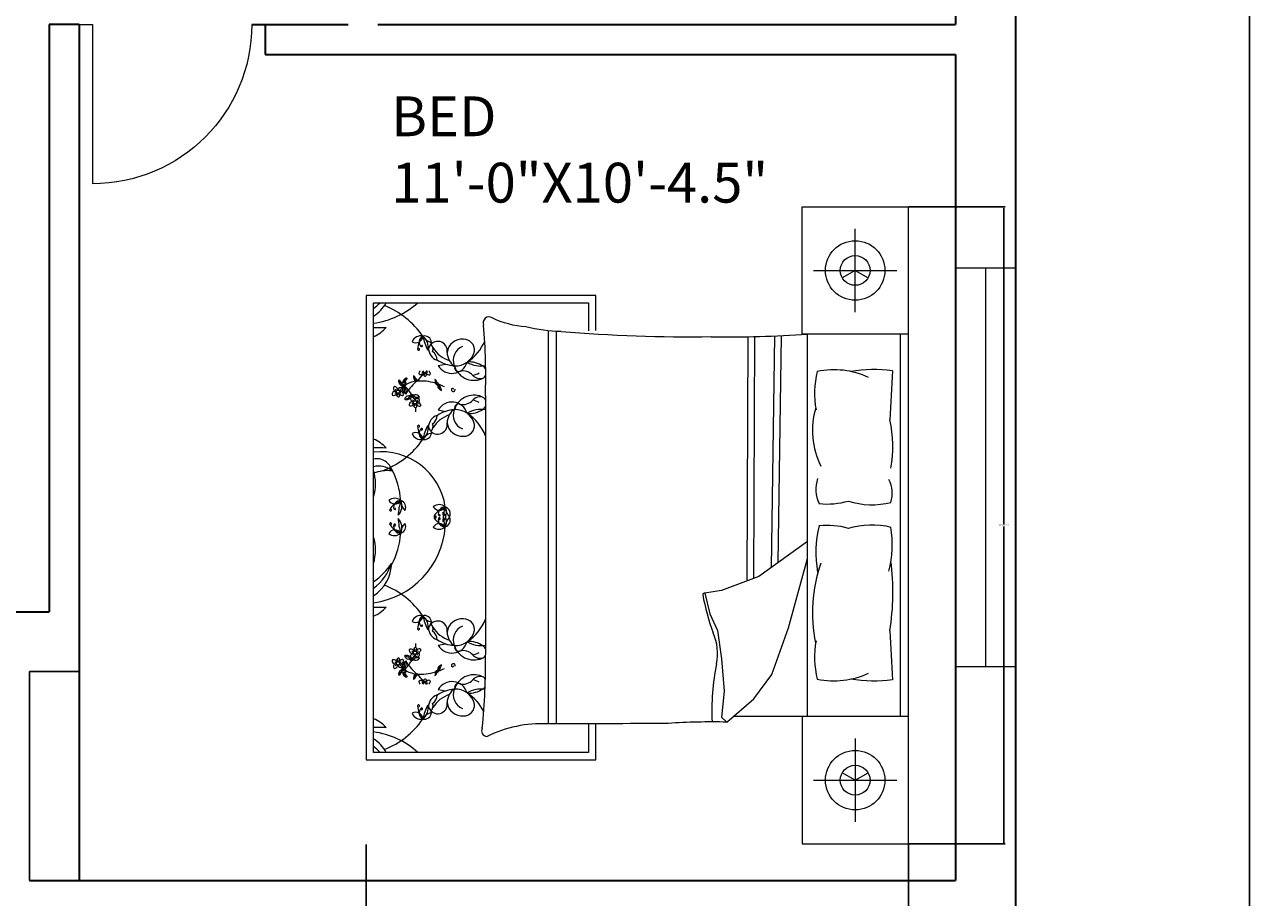
# Model space of a CAD drawing. Units: inches. Extents: x -59 to 444, y -680 to 63.
# Tile 8 of 9: x 260 to 444, y -306 to -175. Entities that reach past the tile are written whole.
import ezdxf

# ---------------------------------------------------------------- set-up
doc = ezdxf.new("R2010")
doc.units = ezdxf.units.IN
doc.header["$MEASUREMENT"] = 0
for name, color, linetype, lineweight in [('A-ANNO-DIMS', 2, 'Continuous', 18), ('A-AREA-IDEN', 7, 'Continuous', 18), ('A-DOOR', 3, 'Continuous', 18), ('A-FLOR-EVTR', 7, 'Continuous', 30), ('A-FURN', 8, 'Continuous', 13), ('A-GLAZ', 4, 'Continuous', 18), ('A-WALL', 7, 'Continuous', 35)]:
    doc.layers.add(name, color=color, linetype=linetype, lineweight=lineweight)
doc.styles.get("Standard").update_dxf_attribs({"font": 'arial.ttf'})
doc.dimstyles.get("Standard").update_dxf_attribs({"dimtxt": 0.18, "dimasz": 0.18, "dimexe": 0.18, "dimexo": 0.0625, "dimgap": 0.09, "dimtad": 0, "dimtih": 1, "dimtoh": 1, "dimdec": 0, "dimzin": 0, "dimdsep": 46, "dimlunit": 3, "dimtxsty": 'Standard', "dimcen": 0.09, "dimadec": 0, "dimazin": 0, "dimtfac": 1, "dimtdec": 0, "dimtofl": 0, "dimtmove": 0, "dimatfit": 3, "dimfxl": 1, "dimtolj": 1, "dimtzin": 0, "dimarcsym": 0})

# ---------------------------------------------------------------- blocks, each defined once
blk = doc.blocks.new('BED-SET-82')
for p, q in [((81.66, 0), (81.66, 96.02)), ((73.65, 80.14), (73.65, 92.69)), ((67.38, 86.42), (79.93, 86.42)), ((0, 82.67), (0, 12.67)), ((34.59, 82.67), (0, 82.67)), ((1.11, 81.56), (33.48, 81.56)), ((1.11, 13.79), (1.11, 81.56)), ((33.48, 81.56), (33.48, 77.33)), ((34.59, 77.35), (34.59, 82.67)), ((27.4, 77.34), (27.4, 18.1)), ((28.6, 77.25), (28.6, 18.1)), ((57.5, 76.47), (57.35, 39.63)), ((58.49, 76.47), (58.34, 40.01)), ((61.51, 76.52), (61.02, 41.65)), ((62.49, 76.56), (62.01, 42.37)), ((66.48, 19.2), (66.48, 76.81)), ((80.42, 76.81), (80.42, 19.2)), ((10.85, 72.1), (11.93, 72.31)), ((17.97, 67.5), (17.97, 28.52)), ((10.85, 65.39), (11.93, 65.18)), ((66.48, 45.58), (59.16, 40.32)), ((63.63, 32.54), (66.48, 43.01)), ((59.16, 40.32), (53.52, 38.18)), ((53.52, 38.18), (51, 37.79)), ((51, 37.79), (51.77, 34.68)), ((51.77, 34.68), (52.94, 32.15)), ((52.94, 32.15), (53.52, 27.87)), ((61.1, 25.54), (63.63, 32.54)), ((10.85, 29.96), (11.93, 30.17)), ((53.52, 27.87), (53.91, 23.01)), ((58.38, 21.84), (61.1, 25.54)), ((10.85, 23.25), (11.93, 23.04)), ((53.91, 23.01), (53.52, 19.12)), ((54.3, 18.34), (58.38, 21.84)), ((53.52, 19.12), (54.3, 18.34)), ((81.66, 19.2), (55.3, 19.2)), ((33.48, 18.1), (33.48, 13.79)), ((34.59, 12.67), (34.59, 18.1)), ((73.65, 15.87), (73.65, 3.33)), ((33.48, 13.79), (1.11, 13.79)), ((0, 12.67), (34.59, 12.67)), ((67.38, 9.6), (79.93, 9.6))]:
    blk.add_line(p, q)
for points in [[(81.66, 76.81), (65.65, 76.81), (65.65, 96.02), (81.66, 96.02)], [(73.65, 86.42), (71.71, 85.3)], [(73.65, 86.42), (75.6, 85.3)], [(65.65, 19.2), (65.65, 0), (81.66, 0)], [(73.65, 9.6), (71.71, 10.72)], [(73.65, 9.6), (75.6, 10.72)]]:
    blk.add_lwpolyline(points)
for points in [[(29.36, 77.22, -0.056112), (24.07, 77.92, -0.095341), (18.98, 79.27)], [(79.26, 71.3, 0.074897), (72.99, 71.18, -0.472817)], [(72.64, 51.66, 0.14099), (79.04, 51.47, 0.235245)], [(72.64, 47.56, -0.14099), (79.04, 47.75, -0.235245)], [(79.26, 24.72, -0.074897), (72.99, 24.83, 0.472817)], [(45.51, 18.14, -0.001242), (27.29, 18.1, 0.127202), (18.21, 16.17)]]:
    blk.add_lwpolyline(points, format="xyb")
for centre, radius in [((73.65, 86.42), 4.48), ((73.65, 86.42), 2.24), ((4.79, 68.15), 0.245), ((7.37, 66.55), 0.245), ((7.37, 28.8), 0.245), ((4.79, 27.2), 0.245), ((73.65, 9.6), 4.48), ((73.65, 9.6), 2.24)]:
    blk.add_circle(centre, radius)
for centre, radius, start, end in [((-2.26, 84.61), 6.11, 303.4617, 330.1116), ((-3.4, 86.8), 7.61, 306.3036, 316.4814), ((-0.58, 90.9), 12.54, 277.745, 311.8856), ((-1.82, 69.44), 12.54, 34.3865, 68.5908), ((-0.84, 81.18), 5.1, 292.5547, 318.9546), ((1.9, 95.15), 17.35, 267.4081, 273.6519), ((18.5, 78.54), 0.875, 56.1736, 203.4781), ((-75.42, 70.44), 93.43, 358.1965, 4.7598), ((8.23, 75.17), 1.39, 77.7115, 159.0387), ((7.48, 76.56), 1.05, 238.4633, 358.2869), ((10.92, 74.44), 3.17, 138.8402, 177.9352), ((9.01, 75.62), 1.03, 117.6827, 223.7762), ((8.78, 75.52), 1.04, 2.9516, 103.728), ((17.09, 78.43), 8.77, 192.5173, 207.1824), ((7.37, 74.92), 1.98, 345.4653, 54.2343), ((10.36, 77.64), 2.14, 211.3827, 255.2969), ((14.47, 73.77), 2.29, 84.9449, 172.8857), ((14.7, 74.43), 1.62, 354.4856, 91.0538), ((48.48, 301.47), 225.05, 265.1265, 270.8855), ((54.75, 248.94), 172.53, 269.0718, 273.9), ((7.9, 74.55), 0.156, 177.9352, 11.4834), ((7.98, 74.56), 0.0756, 11.4834, 127.9409), ((8.42, 75.02), 0.0817, 223.7729, 159.7333), ((11.2, 74.64), 1.8, 175.969, 254.3045), ((10.77, 74.3), 1.44, 350.264, 160.8688), ((9.21, 74.59), 0.883, 333.9755, 53.2681), ((8.81, 72.7), 1.92, 6.1662, 51.5825), ((13.94, 77.15), 4.53, 211.2614, 251.7045), ((14.98, 74.17), 2.79, 182.3591, 234.0401), ((15.34, 72.87), 2.23, 111.5819, 201.4221), ((13.5, 74.93), 2.89, 265.2933, 346.921), ((11.21, 78.67), 7.27, 303.6671, 336.3547), ((13.58, 77.2), 5.15, 236.2883, 266.5076), ((12.92, 73.29), 2.39, 209.9085, 343.1337), ((17.26, 76), 3.98, 238.8218, 280.751), ((15.53, 68.93), 3.7, 55.785, 94.7304), ((9.85, 70.48), 2.71, 178.3264, 187.1302), ((6.92, 70.1), 0.504, 11.3256, 64.4621), ((8.63, 70.83), 1.52, 190.2588, 210.656), ((1.42, 76.4), 9.12, 313.1541, 322.0459), ((8.12, 70.92), 0.188, 142.4737, 265.053), ((8.37, 70.96), 0.404, 127.7621, 169.0403), ((8.15, 71.3), 0.568, 265.053, 338.3618), ((8.91, 70.52), 0.742, 113.4276, 137.6104), ((8.82, 71.29), 0.245, 183.2768, 356.7232), ((9, 70.85), 0.4, 139.7889, 227.6792), ((8.87, 70.71), 0.211, 227.6792, 350.3487), ((8.06, 70.86), 0.801, 353.0852, 15.7171), ((8.58, 70.76), 0.506, 350.3487, 43.6538), ((9.52, 71.28), 0.588, 198.7263, 262.5032), ((9.05, 71.01), 0.234, 1.1081, 91.8675), ((9.49, 70.88), 0.189, 255.2356, 54.9248), ((9.2, 70.95), 0.408, 11.5637, 52.6358), ((13.92, 71.78), 0.596, 167.3041, 285.1471), ((15.53, 68.93), 3.7, 122.7011, 126.3445), ((16.23, 72.92), 3.06, 199.2822, 299.1751), ((14.59, 69.3), 1.97, 41.5653, 105.1471), ((15.67, 73.38), 2.76, 277.436, 299.9149), ((17.14, 71.56), 1.44, 221.5653, 293.8354), ((16.91, 71.07), 1.16, 17.4186, 52.325), ((16.91, 71.07), 1.16, 314.4517, 343.3657), ((80.39, 67.87), 12.87, 165.1039, 191.0369), ((70.47, 59.07), 12.38, 65.1316, 101.7583), ((993.04, 18.37), 915.3, 176.68521, 177.14978), ((4.6, 68.65), 0.483, 157.4086, 261.4386), ((4.33, 68.67), 0.242, 58.0499, 135.6268), ((4.58, 68.51), 0.162, 172.906, 277.132), ((4.05, 68.22), 0.771, 14.7558, 58.0499), ((5.13, 68.42), 0.333, 36.1046, 181.4281), ((5.15, 69.73), 0.273, 124.3538, 214.3923), ((5.55, 69.69), 0.637, 190.3057, 287.1958), ((4.94, 68.68), 0.337, 270.0645, 331.1507), ((5.73, 69.92), 0.739, 176.9701, 248.2913), ((11.01, 73.81), 7.14, 212.6784, 216.3746), ((5.22, 68.46), 0.24, 263.7526, 41.7054), ((5.48, 69.74), 0.283, 216.3746, 291.7548), ((7.98, 65.77), 3.99, 124.0033, 132.4917), ((3.88, 65.27), 4.26, 63.7819, 68.2913), ((6.16, 68.55), 0.678, 128.3208, 208.8162), ((6.16, 69.54), 0.637, 122.8155, 187.3992), ((5.67, 69.28), 0.213, 289.3605, 111.7548), ((5.83, 69.28), 0.213, 221.8703, 44.2646), ((6.79, 68.66), 1.11, 157.2305, 229.0635), ((6.44, 69.46), 0.739, 109.4799, 177.6828), ((6.42, 69.03), 0.656, 174.4544, 220.6188), ((2.69, 65.36), 4.78, 30.544, 49.818), ((6.04, 69.93), 0.273, 56.8636, 146.9021), ((6.18, 69.63), 0.283, 148.8844, 224.2646), ((5.32, 68.09), 0.788, 340.0041, 40.6188), ((12.05, 66.08), 7.14, 145.1882, 148.8844), ((7.98, 65.77), 3.99, 94.756, 119.2041), ((16.47, 60.04), 13.12, 132.2412, 142.1744), ((7.62, 70.21), 0.461, 188.3432, 274.2869), ((8.02, 70.46), 0.805, 210.656, 242.6341), ((8.63, 71.15), 1.54, 218.2101, 226.3071), ((7.49, 69.86), 0.196, 325.7657, 67.4417), ((8.18, 61.81), 7.95, 73.5842, 93.8277), ((13.08, 69.9), 2.71, 178.3264, 187.1302), ((10.15, 69.53), 0.504, 11.3256, 64.4621), ((11.87, 70.25), 1.52, 190.2588, 210.656), ((10.85, 69.64), 0.461, 188.3432, 274.2869), ((11.25, 69.89), 0.805, 210.656, 242.6341), ((11.86, 70.58), 1.54, 218.2101, 226.3071), ((10.72, 69.29), 0.196, 325.7657, 67.4417), ((11.27, 68.93), 0.461, 147.5332, 233.4768), ((11.69, 69.16), 0.805, 179.1859, 211.164), ((10.9, 68.98), 0.196, 354.3784, 96.0543), ((8.18, 61.81), 7.95, 63.0032, 69.8941), ((12.3, 69.53), 1.52, 211.164, 231.5612), ((12.56, 70.77), 2.71, 234.6898, 243.4936), ((12.58, 69.37), 1.54, 195.5129, 203.6099), ((10.85, 68.37), 0.504, 357.3579, 50.4944), ((13.02, 68.47), 0.185, 12.7051, 190.4384), ((13.13, 68.49), 0.301, 190.4384, 10.4136), ((4.09, 67.78), 0.188, 142.4737, 265.053), ((4.34, 67.82), 0.404, 61.2196, 169.0403), ((4.12, 68.16), 0.568, 265.053, 338.3618), ((4.88, 67.38), 0.742, 113.4276, 137.6104), ((4.97, 67.71), 0.4, 139.7889, 227.6792), ((4.84, 67.57), 0.211, 227.6792, 350.3487), ((4.03, 67.71), 0.801, 353.0852, 15.7171), ((4.55, 67.62), 0.506, 350.3487, 43.6538), ((5.49, 68.14), 0.588, 198.7263, 262.5032), ((5.22, 68.6), 0.385, 221.8413, 265.7877), ((5.02, 67.87), 0.234, 1.1081, 91.8675), ((5.17, 67.81), 0.408, 11.5637, 86.365), ((5.46, 67.74), 0.189, 255.2356, 54.9248), ((6.28, 68.6), 0.81, 207.7043, 254.3516), ((5.75, 68.13), 1.11, 270.278, 342.111), ((6.5, 66.74), 0.788, 98.7227, 159.3375), ((6.1, 67.75), 0.81, 244.9899, 291.6373), ((6.28, 68.17), 0.656, 278.7227, 324.8872), ((6.16, 67.64), 0.678, 290.5253, 358.5375), ((6.91, 66.22), 0.404, 61.2196, 169.0403), ((7.18, 67.05), 0.483, 157.4086, 261.4386), ((6.91, 67.07), 0.242, 58.0499, 135.6268), ((7.48, 67.83), 0.678, 182.8499, 266.1226), ((7.22, 68.31), 0.656, 231.7607, 277.9252), ((7.73, 68.42), 1.11, 214.5369, 286.3699), ((7.16, 66.91), 0.162, 172.906, 277.132), ((6.63, 66.62), 0.771, 14.7558, 58.0499), ((2.69, 65.36), 4.78, 23.0501, 23.8477), ((7.42, 66.88), 0.788, 37.3105, 97.9252), ((7.71, 66.82), 0.333, 36.1046, 181.4281), ((7.51, 67.96), 0.81, 265.0106, 311.658), ((7.51, 67.08), 0.337, 270.0645, 331.1507), ((7.8, 67), 0.385, 221.8413, 265.7877), ((7.8, 66.86), 0.24, 263.7526, 41.7054), ((7.75, 66.21), 0.408, 11.5637, 86.365), ((12.92, 64.2), 2.39, 16.8663, 150.0915), ((16.23, 64.57), 3.06, 60.8249, 160.7178), ((14.59, 68.19), 1.97, 254.8529, 318.4347), ((15.67, 64.11), 2.76, 60.0851, 82.564), ((17.14, 65.93), 1.44, 66.1646, 138.4347), ((16.91, 66.41), 1.16, 23.2856, 45.5483), ((6.67, 66.18), 0.188, 142.4737, 265.053), ((6.7, 66.56), 0.568, 265.053, 338.3618), ((7.45, 65.78), 0.742, 113.4276, 137.6104), ((7.55, 66.11), 0.4, 139.7889, 227.6792), ((7.42, 65.97), 0.211, 227.6792, 350.3487), ((6.6, 66.12), 0.801, 353.0852, 15.7171), ((2.69, 65.36), 4.78, 357.1071, 4.7585), ((7.13, 66.02), 0.506, 350.3487, 43.6538), ((8.07, 66.54), 0.588, 198.7263, 262.5032), ((7.6, 66.27), 0.234, 1.1081, 91.8675), ((8.04, 66.14), 0.189, 255.2356, 54.9248), ((13.58, 60.29), 5.15, 93.4924, 123.7117), ((14.98, 63.32), 2.79, 125.9599, 177.6409), ((15.34, 64.62), 2.23, 158.5779, 248.4181), ((13.5, 62.56), 2.89, 13.079, 94.7067), ((13.92, 65.71), 0.596, 74.8529, 192.6959), ((15.53, 68.56), 3.7, 233.6555, 237.2989), ((17.26, 61.49), 3.98, 79.7133, 121.1782), ((15.53, 68.56), 3.7, 265.2696, 304.215), ((11.21, 58.82), 7.27, 21.4941, 56.3329), ((16.91, 66.41), 1.16, 307.675, 336.7144), ((79.44, 62.32), 12.22, 163.8254, 206.1239), ((7.9, 62.94), 0.156, 348.5166, 182.0648), ((10.92, 63.05), 3.17, 182.0648, 221.1598), ((7.98, 62.92), 0.0756, 232.0591, 348.5166), ((7.37, 62.57), 1.98, 305.7657, 14.5347), ((17.09, 59.06), 8.77, 152.8176, 167.4827), ((11.2, 62.85), 1.8, 105.6955, 184.031), ((10.77, 63.19), 1.44, 199.1312, 9.736), ((9.21, 62.9), 0.883, 306.7319, 26.0245), ((8.81, 64.79), 1.92, 308.4175, 353.8338), ((13.94, 60.34), 4.53, 108.2955, 148.7386), ((14.47, 63.72), 2.29, 187.1143, 275.0551), ((14.7, 63.06), 1.62, 268.9462, 5.5144), ((62.46, 59.9), 16.88, 348.8159, 13.6573), ((-0.84, 56.3), 5.1, 41.0454, 67.4453), ((7.48, 60.93), 1.05, 1.7131, 121.5367), ((8.23, 62.32), 1.39, 200.9613, 282.2885), ((9.01, 61.87), 1.03, 136.2238, 242.3173), ((8.36, 62.49), 0.136, 200.2817, 136.2238), ((8.78, 61.97), 1.04, 256.272, 357.0484), ((10.36, 59.85), 2.14, 104.7031, 148.6173), ((1.9, 42.34), 17.35, 86.3481, 92.5919), ((-1.82, 68.04), 12.54, 291.4092, 325.6135), ((2.32, 49.39), 9.7, 8.1803, 97.1364), ((1.64, 55.79), 2.25, 10.9261, 103.6102), ((1.95, 54.1), 2.85, 48.0951, 107.1391), ((-5.48, 54.26), 6.89, 343.5431, 17.0202), ((3.2, 50.64), 5.61, 83.3805, 111.883), ((-7.29, 50.75), 12.54, 4.4623, 27.4146), ((72.82, 53.43), 5.09, 161.4593, 204.9817), ((74.48, 52.78), 4.75, 343.8974, 26.6563), ((-9.03, 51.53), 10.2, 4.3787, 5.6357), ((-16.02, 46.16), 18.22, 19.7217, 19.9028), ((4.27, 50.7), 1.39, 47.7873, 129.1145), ((4.32, 52.28), 1.05, 208.5391, 328.3627), ((3.68, 50.33), 0.156, 148.011, 341.5592), ((6.24, 48.73), 3.17, 108.9159, 148.011), ((3.75, 50.3), 0.0756, 341.5592, 98.0167), ((5.17, 50.7), 1.03, 87.7585, 193.852), ((4.36, 50.48), 0.0817, 193.9791, 129.8091), ((13.58, 49.1), 8.77, 162.593, 177.2582), ((3.4, 50.91), 1.98, 315.5411, 24.3101), ((7.35, 51.78), 2.14, 181.4585, 225.3727), ((4.92, 50.73), 1.04, 333.0274, 73.8037), ((10.99, 49.74), 1.39, 47.7873, 129.1145), ((11.03, 51.32), 1.05, 208.5391, 328.3627), ((12.95, 47.77), 3.17, 108.9159, 148.011), ((11.88, 49.74), 1.03, 87.7585, 193.852), ((10.12, 49.95), 1.98, 315.5411, 24.3101), ((20.29, 48.14), 8.77, 162.593, 177.2582), ((10.12, 48.6), 1.98, 335.6899, 44.4589), ((20.29, 50.4), 8.77, 182.7418, 197.407), ((11.63, 49.77), 1.04, 333.0274, 73.8037), ((14.06, 50.82), 2.14, 181.4585, 225.3727), ((69.43, 62.98), 11.76, 264.0129, 285.8293), ((3.68, 48.22), 0.156, 18.4408, 211.989), ((6.24, 49.82), 3.17, 211.989, 251.0841), ((3.75, 48.25), 0.0756, 261.9833, 18.4408), ((5.17, 47.84), 1.03, 166.148, 272.2415), ((4.3, 48.06), 0.136, 230.0755, 166.148), ((13.58, 49.44), 8.77, 182.7418, 197.407), ((3.4, 47.64), 1.98, 335.6899, 44.4589), ((7.35, 46.76), 2.14, 134.6273, 178.5415), ((4.92, 47.82), 1.04, 286.1963, 26.9726), ((11.03, 47.23), 1.05, 31.6373, 151.4609), ((10.39, 49.37), 0.156, 148.011, 341.5592), ((10.39, 49.18), 0.156, 18.4408, 211.989), ((12.95, 50.78), 3.17, 211.989, 251.0841), ((10.47, 49.34), 0.0756, 341.5592, 98.0167), ((10.47, 49.21), 0.0756, 261.9833, 18.4408), ((11.88, 48.8), 1.03, 166.148, 272.2415), ((11.02, 49.02), 0.136, 230.0755, 166.148), ((11.07, 49.52), 0.0817, 193.9791, 129.8091), ((11.63, 48.78), 1.04, 286.1963, 26.9726), ((14.06, 47.73), 2.14, 134.6273, 178.5415), ((-0.58, 48.76), 12.54, 277.745, 355.5377), ((-5.48, 44.29), 6.89, 342.9798, 16.4569), ((-9.03, 47.02), 10.2, 354.3643, 355.6213), ((-16.02, 52.39), 18.22, 340.0972, 340.2783), ((4.32, 46.27), 1.05, 31.6373, 151.4609), ((4.27, 47.85), 1.39, 230.8855, 312.2127), ((-7.29, 47.8), 12.54, 332.5854, 355.5377), ((10.99, 48.81), 1.39, 230.8855, 312.2127), ((84.66, 43.95), 16.93, 166.3762, 190.1383), ((69.43, 36.24), 11.76, 74.1707, 95.9871), ((62.12, 45.23), 17.11, 346.04, 8.4751), ((44.52, 37.87), 34.82, 350.503, 7.7804), ((-2.26, 42.46), 6.11, 303.4617, 358.728), ((-5.54, 48.66), 11.33, 305.947, 325.9877), ((-3.4, 44.66), 7.61, 306.3036, 342.1496), ((89.53, 34.92), 22.32, 160.7385, 191.9603), ((-1.82, 27.3), 12.54, 34.3865, 68.5908), ((50.92, 37.57), 0.232, 70.2464, 181.1377), ((87.28, 44.46), 37.24, 190.6617, 199.8806), ((1.9, 53.01), 17.35, 267.4081, 273.6519), ((-0.84, 39.04), 5.1, 292.5547, 318.9546), ((8.23, 33.03), 1.39, 77.7115, 159.0387), ((7.48, 34.42), 1.05, 238.4633, 358.2869), ((10.92, 32.3), 3.17, 138.8402, 177.9352), ((9.01, 33.48), 1.03, 117.6827, 223.7762), ((8.78, 33.38), 1.04, 2.9516, 103.728), ((10.36, 35.5), 2.14, 211.3827, 255.2969), ((7.37, 32.78), 1.98, 345.4653, 54.2343), ((17.09, 36.29), 8.77, 192.5173, 207.1824), ((10.77, 32.15), 1.44, 350.264, 160.8688), ((14.47, 31.63), 2.29, 84.9449, 172.8857), ((14.7, 32.29), 1.62, 354.4856, 91.0538), ((11.21, 36.52), 7.27, 303.6671, 338.5059), ((7.9, 32.41), 0.156, 177.9352, 11.4834), ((7.98, 32.42), 0.0756, 11.4834, 127.9409), ((8.42, 32.88), 0.0817, 223.7729, 159.7333), ((11.2, 32.5), 1.8, 175.969, 254.3045), ((9.21, 32.45), 0.883, 333.9755, 53.2681), ((8.81, 30.56), 1.92, 6.1662, 51.5825), ((13.94, 35.01), 4.53, 211.2614, 251.7045), ((14.98, 32.03), 2.79, 182.3591, 234.0401), ((15.34, 30.72), 2.23, 111.5819, 201.4221), ((13.5, 32.79), 2.89, 265.2933, 346.921), ((45.11, 28.65), 7.82, 348.6608, 23.7384), ((993.04, 77.64), 915.3, 182.85022, 183.31479), ((7.42, 29.38), 0.211, 9.6513, 132.3208), ((2.69, 29.98), 4.78, 355.2415, 2.8929), ((13.58, 35.05), 5.15, 236.2883, 266.5076), ((12.92, 31.15), 2.39, 209.9085, 343.1337), ((13.92, 29.64), 0.596, 167.3041, 285.1471), ((15.53, 26.79), 3.7, 122.7011, 126.3445), ((16.23, 30.78), 3.06, 199.2822, 299.1751), ((17.26, 33.86), 3.98, 238.8218, 280.2867), ((15.53, 26.79), 3.7, 55.785, 94.7304), ((16.91, 28.93), 1.16, 23.2856, 52.325), ((80.39, 28.14), 12.87, 168.9631, 194.8961), ((4.09, 27.57), 0.188, 94.947, 217.5263), ((4.12, 27.19), 0.568, 21.6382, 94.947), ((4.97, 27.64), 0.4, 132.3208, 220.2111), ((4.84, 27.78), 0.211, 9.6513, 132.3208), ((4.03, 27.63), 0.801, 344.2829, 6.9148), ((4.55, 27.73), 0.506, 316.3462, 9.6513), ((5.49, 27.21), 0.588, 97.4968, 161.2737), ((5.46, 27.61), 0.189, 305.0752, 104.7644), ((6.1, 27.59), 0.81, 68.3627, 115.0101), ((5.75, 27.21), 1.11, 17.889, 89.722), ((6.5, 28.61), 0.788, 200.6625, 261.2773), ((6.28, 27.18), 0.656, 35.1128, 81.2773), ((6.16, 27.71), 0.678, 1.4625, 69.4747), ((6.67, 29.17), 0.188, 94.947, 217.5263), ((6.91, 29.13), 0.404, 190.9597, 298.7804), ((6.7, 28.79), 0.568, 21.6382, 94.947), ((7.18, 28.3), 0.483, 98.5614, 202.5914), ((6.91, 28.28), 0.242, 224.3732, 301.9501), ((7.48, 27.52), 0.678, 93.8774, 177.1501), ((7.73, 26.92), 1.11, 73.6301, 145.4631), ((7.45, 29.56), 0.742, 222.3896, 246.5724), ((7.16, 28.43), 0.162, 82.868, 187.094), ((6.63, 28.73), 0.771, 301.9501, 345.2442), ((2.69, 29.98), 4.78, 336.1523, 336.9499), ((7.55, 29.24), 0.4, 132.3208, 220.2111), ((7.42, 28.47), 0.788, 262.0748, 322.6895), ((6.6, 29.23), 0.801, 344.2829, 6.9148), ((7.71, 28.53), 0.333, 178.5719, 323.8954), ((7.51, 27.39), 0.81, 48.342, 94.9894), ((7.13, 29.33), 0.506, 316.3462, 9.6513), ((8.07, 28.81), 0.588, 97.4968, 161.2737), ((7.8, 28.34), 0.385, 94.2123, 138.1587), ((7.51, 28.26), 0.337, 28.8493, 89.9355), ((7.6, 29.08), 0.234, 268.1325, 358.8919), ((7.75, 29.13), 0.408, 273.635, 348.4363), ((7.8, 28.49), 0.24, 318.2946, 96.2474), ((8.04, 29.21), 0.189, 305.0752, 104.7644), ((14.59, 27.16), 1.97, 41.5653, 105.1471), ((15.67, 31.24), 2.76, 277.436, 299.9149), ((17.14, 29.42), 1.44, 221.5653, 293.8354), ((-81.98, 27.37), 99.96, 354.3113, 0.6567), ((16.91, 28.93), 1.16, 314.4517, 336.771), ((4.34, 27.53), 0.404, 190.9597, 298.7804), ((4.6, 26.7), 0.483, 98.5614, 202.5914), ((4.33, 26.68), 0.242, 224.3732, 301.9501), ((4.88, 27.96), 0.742, 222.3896, 246.5724), ((4.58, 26.83), 0.162, 82.868, 187.094), ((4.05, 27.13), 0.771, 301.9501, 345.2442), ((5.13, 26.93), 0.333, 178.5719, 323.8954), ((5.55, 25.66), 0.637, 72.8042, 169.6943), ((5.22, 26.74), 0.385, 94.2123, 138.1587), ((4.94, 26.66), 0.337, 28.8493, 89.9355), ((5.73, 25.43), 0.739, 111.7087, 183.0299), ((5.02, 27.48), 0.234, 268.1325, 358.8919), ((5.17, 27.53), 0.408, 273.635, 348.4363), ((5.22, 26.89), 0.24, 318.2946, 96.2474), ((5.48, 25.6), 0.283, 68.2452, 143.6254), ((7.98, 29.57), 3.99, 227.5083, 235.9967), ((3.88, 30.08), 4.26, 291.7087, 296.2181), ((6.16, 26.8), 0.678, 151.1838, 231.6792), ((6.16, 25.8), 0.637, 172.6008, 237.1845), ((6.28, 26.75), 0.81, 105.6484, 152.2957), ((5.67, 26.07), 0.213, 248.2452, 70.6395), ((5.83, 26.07), 0.213, 315.7354, 138.1297), ((6.79, 26.69), 1.11, 130.9365, 202.7695), ((6.42, 26.32), 0.656, 139.3812, 185.5456), ((2.69, 29.98), 4.78, 310.182, 329.456), ((6.18, 25.72), 0.283, 135.7354, 211.1156), ((5.32, 27.26), 0.788, 319.3812, 19.9959), ((7.98, 29.57), 3.99, 240.7959, 265.244), ((16.47, 35.31), 13.12, 217.8256, 227.7588), ((7.22, 27.04), 0.656, 82.0748, 128.2393), ((8.18, 33.53), 7.95, 266.1723, 286.4158), ((10.85, 25.71), 0.461, 85.7131, 171.6568), ((11.25, 25.46), 0.805, 117.3659, 149.344), ((11.86, 24.77), 1.54, 133.6929, 141.7899), ((10.72, 26.06), 0.196, 292.5583, 34.2343), ((11.27, 26.42), 0.461, 126.5232, 212.4668), ((11.69, 26.18), 0.805, 148.836, 180.8141), ((10.9, 26.37), 0.196, 263.9457, 5.6216), ((8.18, 33.53), 7.95, 290.1059, 296.9968), ((12.3, 25.81), 1.52, 128.4388, 148.836), ((12.56, 24.58), 2.71, 116.5064, 125.3102), ((12.58, 25.97), 1.54, 156.3901, 164.4871), ((10.85, 26.98), 0.504, 309.5056, 2.6421), ((13.13, 26.86), 0.301, 349.5864, 169.5616), ((13.02, 26.88), 0.185, 169.5616, 347.2949), ((88.3, 19.99), 36.24, 168.6608, 182.5481), ((5.15, 25.62), 0.273, 145.6077, 235.6462), ((11.01, 21.54), 7.14, 143.6254, 147.3216), ((6.44, 25.88), 0.739, 182.3172, 250.5201), ((6.04, 25.42), 0.273, 213.0979, 303.1364), ((12.05, 29.27), 7.14, 211.1156, 214.8118), ((8.63, 24.52), 1.52, 149.344, 169.7412), ((9.85, 24.87), 2.71, 172.8698, 181.6736), ((6.92, 25.25), 0.504, 295.5379, 348.6744), ((7.62, 25.14), 0.461, 85.7131, 171.6568), ((8.02, 24.88), 0.805, 117.3659, 149.344), ((8.63, 24.19), 1.54, 133.6929, 141.7899), ((7.49, 25.49), 0.196, 292.5583, 34.2343), ((1.42, 18.95), 9.12, 37.9541, 46.8459), ((8.12, 24.43), 0.188, 94.947, 217.5263), ((8.37, 24.39), 0.404, 190.9597, 232.2379), ((8.15, 24.05), 0.568, 21.6382, 94.947), ((8.91, 24.82), 0.742, 222.3896, 246.5724), ((8.82, 24.05), 0.245, 3.2768, 176.7232), ((9, 24.5), 0.4, 132.3208, 220.2111), ((8.87, 24.64), 0.211, 9.6513, 132.3208), ((8.06, 24.49), 0.801, 344.2829, 6.9148), ((8.58, 24.59), 0.506, 316.3462, 9.6513), ((9.52, 24.07), 0.588, 97.4968, 161.2737), ((9.05, 24.34), 0.234, 268.1325, 358.8919), ((9.49, 24.47), 0.189, 305.0752, 104.7644), ((9.2, 24.39), 0.408, 307.3642, 348.4363), ((11.87, 25.09), 1.52, 149.344, 169.7412), ((13.08, 25.44), 2.71, 172.8698, 181.6736), ((10.15, 25.82), 0.504, 295.5379, 348.6744), ((12.92, 22.06), 2.39, 16.8663, 150.0915), ((13.92, 23.57), 0.596, 74.8529, 192.6959), ((16.23, 22.43), 3.06, 60.8249, 160.7178), ((14.59, 26.04), 1.97, 254.8529, 318.4347), ((15.67, 21.97), 2.76, 60.0851, 82.564), ((17.14, 23.79), 1.44, 66.1646, 138.4347), ((16.91, 24.27), 1.16, 26.442, 45.5483), ((70.47, 36.95), 12.38, 258.2417, 294.8684), ((11.2, 20.71), 1.8, 105.6955, 184.031), ((8.81, 22.64), 1.92, 308.4175, 353.8338), ((13.94, 18.19), 4.53, 108.2955, 148.7386), ((13.58, 18.15), 5.15, 93.4924, 123.7117), ((14.98, 21.18), 2.79, 125.9599, 177.6409), ((15.34, 22.48), 2.23, 158.5779, 248.4181), ((13.5, 20.42), 2.89, 13.079, 94.7067), ((15.53, 26.42), 3.7, 233.6555, 237.2989), ((17.26, 19.35), 3.98, 80.8446, 121.1782), ((15.53, 26.42), 3.7, 265.2696, 304.215), ((11.21, 16.68), 7.27, 26.7003, 56.3329), ((16.91, 24.27), 1.16, 307.675, 329.9707), ((7.9, 20.8), 0.156, 348.5166, 182.0648), ((10.92, 20.91), 3.17, 182.0648, 221.1598), ((7.98, 20.78), 0.0756, 232.0591, 348.5166), ((9.01, 19.73), 1.03, 136.2238, 242.3173), ((8.36, 20.35), 0.136, 200.2817, 136.2238), ((17.09, 16.92), 8.77, 152.8176, 167.4827), ((7.37, 20.43), 1.98, 305.7657, 14.5347), ((10.77, 21.05), 1.44, 199.1312, 9.736), ((9.21, 20.75), 0.883, 306.7319, 26.0245), ((14.47, 21.58), 2.29, 187.1143, 275.0551), ((14.7, 20.91), 1.62, 268.9462, 5.5144), ((-0.84, 14.16), 5.1, 41.0454, 67.4453), ((-1.82, 25.9), 12.54, 291.4092, 325.6135), ((7.48, 18.79), 1.05, 1.7131, 121.5367), ((8.23, 20.18), 1.39, 200.9613, 282.2885), ((10.36, 17.71), 2.14, 104.7031, 148.6173), ((8.78, 19.83), 1.04, 256.272, 357.0484), ((1.9, 0.2), 17.35, 86.3481, 92.5919), ((-0.58, 4.45), 12.54, 48.1144, 82.255), ((18.27, 17.06), 0.886, 152.6588, 266.02), ((51.91, -69.69), 88.07, 88.447, 94.1706), ((-2.26, 10.74), 6.11, 29.8884, 56.5383), ((-3.4, 8.54), 7.61, 43.5186, 53.6964)]:
    blk.add_arc(centre, radius, start, end)
blk = doc.blocks.new('WIN-60-W9')
for p, q in [((60, 9), (0, 9)), ((0, 9), (0, 0)), ((60, 0), (60, 9)), ((0, 4.5), (60, 4.5)), ((0, 0), (60, 0))]:
    blk.add_line(p, q)
blk = doc.blocks.new('DOOR-SWING-24')
blk.add_line((24, 0), (0, 0))
blk.add_arc((24, 0), 24, 90, 180)
blk = doc.blocks.new('*D38')
at = {"layer": 'A-ANNO-DIMS', "color": 0, "lineweight": -2, "transparency": 16777216}
for p, q in [((392.67, -202.41), (407.19, -202.41)), ((407.01, -202.59), (407.01, -250.23)), ((407.01, -298.24), (407.01, -250.6)), ((392.67, -298.42), (407.19, -298.42))]:
    blk.add_line(p, q, dxfattribs=at)
at = {"layer": 'A-ANNO-DIMS', "color": 0, "transparency": 16777216}
for points in [[(406.98, -202.59), (407.04, -202.59), (407.01, -202.41)], [(406.98, -298.24), (407.04, -298.24), (407.01, -298.42)]]:
    blk.add_solid(points, dxfattribs=at)
at = {"layer": 'Defpoints', "color": 0, "transparency": 16777216}
for p in [(392.61, -202.41), (407.01, -202.41), (392.61, -298.42)]:
    blk.add_point(p, dxfattribs=at)
at = {"layer": 'A-ANNO-DIMS', "color": 0, "transparency": 16777216, "insert": (407.01, -250.41), "char_height": 0.18, "attachment_point": 5}
blk.add_mtext('\\A1;BED C 96 TYP.', dxfattribs=at)
blk = doc.blocks.new('*D39')
at = {"layer": 'A-ANNO-DIMS', "color": 0, "lineweight": -2, "transparency": 16777216}
for p, q in [((310.95, -298.49), (310.95, -313.01)), ((392.61, -298.49), (392.61, -313.01)), ((311.13, -312.83), (351.25, -312.83)), ((392.43, -312.83), (352.31, -312.83))]:
    blk.add_line(p, q, dxfattribs=at)
at = {"layer": 'A-ANNO-DIMS', "color": 0, "transparency": 16777216}
for points in [[(311.13, -312.8), (311.13, -312.86), (310.95, -312.83)], [(392.43, -312.8), (392.43, -312.86), (392.61, -312.83)]]:
    blk.add_solid(points, dxfattribs=at)
at = {"layer": 'Defpoints', "color": 0, "transparency": 16777216}
for p in [(310.95, -298.42), (392.61, -298.42), (392.61, -312.83)]:
    blk.add_point(p, dxfattribs=at)
at = {"layer": 'A-ANNO-DIMS', "color": 0, "transparency": 16777216, "insert": (351.78, -312.83), "char_height": 0.18, "attachment_point": 5}
blk.add_mtext('\\A1;82 TYP.', dxfattribs=at)
blk = doc.blocks.new('*D47')
at = {"layer": 'A-ANNO-DIMS', "color": 0, "lineweight": -2, "transparency": 16777216}
for p, q in [((267.79, 27.31), (444.16, 27.31)), ((443.98, 27.13), (443.98, -308.38)), ((443.98, -644.26), (443.98, -308.74)), ((267.79, -644.44), (444.16, -644.44))]:
    blk.add_line(p, q, dxfattribs=at)
at = {"layer": 'A-ANNO-DIMS', "color": 0, "transparency": 16777216}
for points in [[(443.95, 27.13), (444.01, 27.13), (443.98, 27.31)], [(443.95, -644.26), (444.01, -644.26), (443.98, -644.44)]]:
    blk.add_solid(points, dxfattribs=at)
at = {"layer": 'Defpoints', "color": 0, "transparency": 16777216}
for p in [(267.73, 27.31), (443.98, 27.31), (267.73, -644.44)]:
    blk.add_point(p, dxfattribs=at)
at = {"layer": 'A-ANNO-DIMS', "color": 0, "transparency": 16777216, "insert": (443.98, -308.56), "char_height": 0.18, "attachment_point": 5}
blk.add_mtext('\\A1;671.8', dxfattribs=at)

msp = doc.modelspace()

# ---------------------------------------------------------------- linework, layer by layer
at = {"layer": 'A-DOOR'}
msp.add_line((267.73, -174.94), (269.73, -174.94), dxfattribs=at)
at = {"layer": 'A-FLOR-EVTR'}
for q in [(260.23, -303.94), (267.73, -272.44)]:
    msp.add_line((260.23, -272.44), q, dxfattribs=at)
at = {"layer": 'A-WALL'}
for p, q in [((408.73, 15.56), (408.73, -632.44)), ((399.73, -126.94), (399.73, -174.94)), ((267.73, -174.94), (263.23, -174.94)), ((263.23, -174.94), (263.23, -263.44)), ((267.73, -174.94), (267.73, -303.94)), ((293.73, -174.94), (308.23, -174.94)), ((295.73, -174.94), (295.73, -179.44)), ((312.73, -174.94), (399.73, -174.94)), ((295.73, -179.44), (399.73, -179.44)), ((399.73, -179.44), (399.73, -303.94)), ((159.23, -263.44), (263.23, -263.44)), ((260.23, -303.94), (399.73, -303.94))]:
    msp.add_line(p, q, dxfattribs=at)

# ---------------------------------------------------------------- block references
at = {"layer": 'A-DOOR', "extrusion": (0, 0, -1), "zscale": -1, "rotation": 89.99999999999996}
msp.add_blockref('DOOR-SWING-24', (-269.73, -198.94), dxfattribs=at)
at = {"layer": 'A-FURN'}
msp.add_blockref('BED-SET-82', (310.95, -298.42), dxfattribs=at)
at = {"layer": 'A-GLAZ', "rotation": 269.9999999999999}
msp.add_blockref('WIN-60-W9', (399.73, -211.68), dxfattribs=at)

# ---------------------------------------------------------------- texts
at = {"layer": 'A-AREA-IDEN', "insert": (314.74, -185.77), "char_height": 6, "attachment_point": 1}
msp.add_mtext('BED\\P11\'-0"X10\'-4.5"', dxfattribs=at)

# ---------------------------------------------------------------- dimensions: what is measured, and where the dimension line sits
at = {"layer": 'A-ANNO-DIMS'}
dim = msp.add_linear_dim(base=(443.9798, 27.314705), p1=(267.7298, -644.435295), p2=(267.7298, 27.314705), angle=90, dimstyle='Standard', override={"dimdec": 1, "dimlfac": 1, "dimrnd": 0, "dimzin": 0, "dimdsep": 46, "dimlunit": 2}, dxfattribs=at)
dim.commit()
dim.dimension.update_dxf_attribs({"geometry": '*D47', "text_midpoint": (443.9798, -308.560295)})
dim = msp.add_linear_dim(base=(407.01, -202.41), p1=(392.61, -298.42), p2=(392.61, -202.41), angle=90, text='BED C <> TYP.', dimstyle='Standard', override={"dimdec": 0, "dimlfac": 1, "dimrnd": 0, "dimzin": 0, "dimdsep": 46, "dimlunit": 2}, dxfattribs=at)
dim.commit()
dim.dimension.update_dxf_attribs({"geometry": '*D38', "text_midpoint": (407.01, -250.41)})
dim = msp.add_linear_dim(base=(392.61, -312.83), p1=(310.95, -298.42), p2=(392.61, -298.42), text='<> TYP.', dimstyle='Standard', override={"dimdec": 0, "dimlfac": 1, "dimrnd": 0, "dimzin": 0, "dimdsep": 46, "dimlunit": 2}, dxfattribs=at)
dim.commit()
dim.dimension.update_dxf_attribs({"geometry": '*D39', "text_midpoint": (351.78, -312.83)})

doc.saveas('drawing.dxf')
